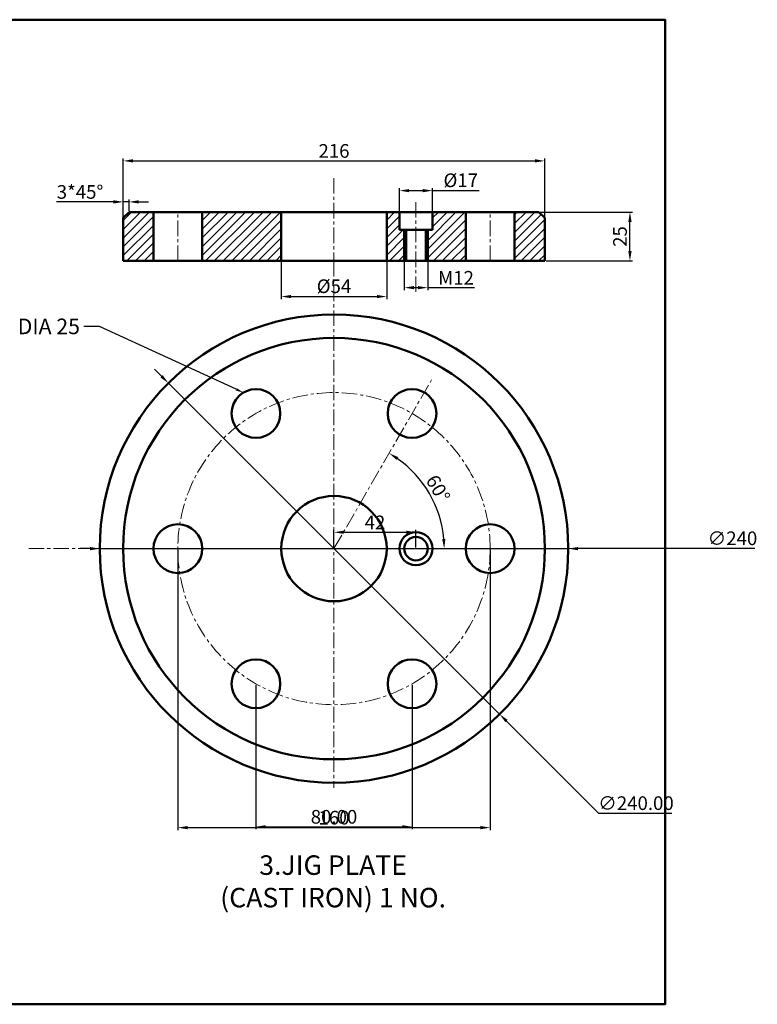
# Model space of a CAD drawing. Units: millimetres. Extents: x 51 to 972, y -225 to 280.
# Tile 3 of 3: x 594 to 972, y -225 to 280. Entities that reach past the tile are written whole.
import ezdxf
from ezdxf import colors
from ezdxf.entities.mleader import LeaderData, LeaderLine
from ezdxf.math import Vec2, Vec3

# ---------------------------------------------------------------- set-up
doc = ezdxf.new("R2010")
doc.units = ezdxf.units.MM
doc.header["$LTSCALE"] = 0.5
doc.linetypes.add('CENTER', pattern=[50.8, 31.75, -6.35, 6.35, -6.35])
for name, color, linetype, lineweight in [('M-CNTR', 1, 'CENTER', 18), ('M-DIMS', 2, 'Continuous', 25), ('M-HATC', 8, 'Continuous', 18), ('M-OUTL', 7, 'Continuous', 50), ('M-TEXT', 7, 'Continuous', 25), ('M-TTLB', 7, 'Continuous', 50)]:
    doc.layers.add(name, color=color, linetype=linetype, lineweight=lineweight)
doc.styles.get("Standard").update_dxf_attribs({"font": 'arial.ttf'})
doc.dimstyles.new('ISO-25', dxfattribs={"dimtxt": 7, "dimasz": 5, "dimexe": 1.25, "dimexo": 0.625, "dimtad": 1, "dimtoh": 1, "dimtxsty": 'Standard', "dimcen": 2.5, "dimadec": 0, "dimazin": 0, "dimtfac": 1, "dimtmove": 0, "dimatfit": 3, "dimfxl": 1, "dimarcsym": 0})

# ---------------------------------------------------------------- blocks, each defined once
blk = doc.blocks.new('*D37')
at = {"layer": 'Defpoints', "color": 0, "ltscale": 0.5, "transparency": 16777216}
for p in [(728.45, 156.09), (782.45, 156.09), (782.45, 137.8)]:
    blk.add_point(p, dxfattribs=at)
at = {"layer": 'M-DIMS', "color": 0, "lineweight": -2, "ltscale": 0.5, "transparency": 16777216}
for p, q in [((728.45, 155.46), (728.45, 136.55)), ((782.45, 155.46), (782.45, 136.55)), ((733.45, 137.8), (777.45, 137.8))]:
    blk.add_line(p, q, dxfattribs=at)
at = {"layer": 'M-DIMS', "color": 0, "ltscale": 0.5, "transparency": 16777216}
for points in [[(733.45, 138.64), (733.45, 136.97), (728.45, 137.8)], [(777.45, 138.64), (777.45, 136.97), (782.45, 137.8)]]:
    blk.add_solid(points, dxfattribs=at)
at = {"layer": 'M-DIMS', "color": 0, "ltscale": 0.5, "transparency": 16777216, "insert": (755.45, 142.2), "char_height": 7, "attachment_point": 5}
blk.add_mtext('%%C54', dxfattribs=at)
blk = doc.blocks.new('*D38')
at = {"layer": 'Defpoints', "color": 0, "ltscale": 0.5, "transparency": 16777216}
for p in [(675.45, 8.59), (835.45, 8.59), (835.45, -134.43)]:
    blk.add_point(p, dxfattribs=at)
at = {"layer": 'M-DIMS', "color": 0, "lineweight": -2, "ltscale": 0.5, "transparency": 16777216}
for p, q in [((675.45, 7.97), (675.45, -135.68)), ((835.45, 7.97), (835.45, -135.68)), ((680.45, -134.43), (830.45, -134.43))]:
    blk.add_line(p, q, dxfattribs=at)
at = {"layer": 'M-DIMS', "color": 0, "ltscale": 0.5, "transparency": 16777216}
for points in [[(680.45, -133.6), (680.45, -135.27), (675.45, -134.43)], [(830.45, -133.6), (830.45, -135.27), (835.45, -134.43)]]:
    blk.add_solid(points, dxfattribs=at)
at = {"layer": 'M-DIMS', "color": 0, "ltscale": 0.5, "transparency": 16777216, "insert": (755.45, -130.23), "char_height": 7, "attachment_point": 5}
blk.add_mtext('160', dxfattribs=at)
blk = doc.blocks.new('*D39')
at = {"layer": 'Defpoints', "color": 0, "ltscale": 0.5, "transparency": 16777216}
for p in [(797.45, 16.98), (755.45, 8.59), (797.45, 8.59)]:
    blk.add_point(p, dxfattribs=at)
at = {"layer": 'M-DIMS', "color": 0, "lineweight": -2, "ltscale": 0.5, "transparency": 16777216}
for p, q in [((755.45, 9.22), (755.45, 18.23)), ((760.45, 16.98), (792.45, 16.98)), ((797.45, 9.22), (797.45, 18.23))]:
    blk.add_line(p, q, dxfattribs=at)
at = {"layer": 'M-DIMS', "color": 0, "ltscale": 0.5, "transparency": 16777216}
for points in [[(760.45, 17.81), (760.45, 16.14), (755.45, 16.98)], [(792.45, 17.81), (792.45, 16.14), (797.45, 16.98)]]:
    blk.add_solid(points, dxfattribs=at)
at = {"layer": 'M-DIMS', "color": 0, "ltscale": 0.5, "transparency": 16777216, "insert": (776.45, 21.12), "char_height": 7, "attachment_point": 5}
blk.add_mtext('42', dxfattribs=at)
blk = doc.blocks.new('*D40')
at = {"layer": 'Defpoints', "color": 0, "ltscale": 0.5, "transparency": 16777216}
for p in [(805.93, 96.03), (808.52, 27.91), (599.02, 8.59), (755.45, 8.59), (887.08, 8.59)]:
    blk.add_point(p, dxfattribs=at)
at = {"layer": 'M-DIMS', "color": 0, "lineweight": -2, "ltscale": 0.5, "transparency": 16777216}
blk.add_arc((755.45, 8.59), 56.47, 5.0746, 54.9254, dxfattribs=at)
at = {"layer": 'M-DIMS', "color": 0, "ltscale": 0.5, "transparency": 16777216}
for points in [[(787.45, 54.11), (788.35, 55.51), (783.69, 57.5)], [(812.53, 13.62), (810.87, 13.55), (811.92, 8.59)]]:
    blk.add_solid(points, dxfattribs=at)
at = {"layer": 'M-DIMS', "color": 0, "ltscale": 0.5, "transparency": 16777216, "insert": (807.99, 38.93), "char_height": 7, "attachment_point": 5, "rotation": 300}
blk.add_mtext('60°', dxfattribs=at)
blk = doc.blocks.new('*D41')
at = {"layer": 'Defpoints', "color": 0, "ltscale": 0.5, "transparency": 16777216}
for p in [(863.45, 207.35), (647.45, 167.09), (863.45, 167.09)]:
    blk.add_point(p, dxfattribs=at)
at = {"layer": 'M-DIMS', "color": 0, "lineweight": -2, "ltscale": 0.5, "transparency": 16777216}
for p, q in [((647.45, 167.71), (647.45, 208.6)), ((652.45, 207.35), (858.45, 207.35)), ((863.45, 167.71), (863.45, 208.6))]:
    blk.add_line(p, q, dxfattribs=at)
at = {"layer": 'M-DIMS', "color": 0, "ltscale": 0.5, "transparency": 16777216}
for points in [[(652.45, 208.19), (652.45, 206.52), (647.45, 207.35)], [(858.45, 208.19), (858.45, 206.52), (863.45, 207.35)]]:
    blk.add_solid(points, dxfattribs=at)
at = {"layer": 'M-DIMS', "color": 0, "ltscale": 0.5, "transparency": 16777216, "insert": (755.45, 211.55), "char_height": 7, "attachment_point": 5}
blk.add_mtext('216', dxfattribs=at)
blk = doc.blocks.new('*D42')
at = {"layer": 'Defpoints', "color": 0, "ltscale": 0.5, "transparency": 16777216}
for p in [(791.45, 156.09), (803.45, 156.09), (803.45, 142.37)]:
    blk.add_point(p, dxfattribs=at)
at = {"layer": 'M-DIMS', "color": 0, "lineweight": -2, "ltscale": 0.5, "transparency": 16777216}
for p, q in [((791.45, 155.46), (791.45, 141.12)), ((803.45, 155.46), (803.45, 141.12)), ((796.45, 142.37), (798.45, 142.37)), ((803.45, 142.37), (827.48, 142.37))]:
    blk.add_line(p, q, dxfattribs=at)
at = {"layer": 'M-DIMS', "color": 0, "ltscale": 0.5, "transparency": 16777216}
for points in [[(796.45, 143.21), (796.45, 141.54), (791.45, 142.37)], [(798.45, 143.21), (798.45, 141.54), (803.45, 142.37)]]:
    blk.add_solid(points, dxfattribs=at)
at = {"layer": 'M-DIMS', "color": 0, "ltscale": 0.5, "transparency": 16777216, "insert": (817.97, 146.51), "char_height": 7, "attachment_point": 5}
blk.add_mtext('M12', dxfattribs=at)
blk = doc.blocks.new('*D43')
at = {"layer": 'Defpoints', "color": 0, "ltscale": 0.5, "transparency": 16777216}
for p in [(805.95, 192.1), (788.95, 181.09), (805.95, 181.09)]:
    blk.add_point(p, dxfattribs=at)
at = {"layer": 'M-DIMS', "color": 0, "lineweight": -2, "ltscale": 0.5, "transparency": 16777216}
for p, q in [((788.95, 181.71), (788.95, 193.35)), ((793.95, 192.1), (800.95, 192.1)), ((805.95, 181.71), (805.95, 193.35)), ((805.95, 192.1), (829.84, 192.1))]:
    blk.add_line(p, q, dxfattribs=at)
at = {"layer": 'M-DIMS', "color": 0, "ltscale": 0.5, "transparency": 16777216}
for points in [[(793.95, 192.93), (793.95, 191.27), (788.95, 192.1)], [(800.95, 192.93), (800.95, 191.27), (805.95, 192.1)]]:
    blk.add_solid(points, dxfattribs=at)
at = {"layer": 'M-DIMS', "color": 0, "ltscale": 0.5, "transparency": 16777216, "insert": (820.4, 196.49), "char_height": 7, "attachment_point": 5}
blk.add_mtext('%%C17', dxfattribs=at)
blk = doc.blocks.new('*D44')
at = {"layer": 'Defpoints', "color": 0, "ltscale": 0.5, "transparency": 16777216}
for p in [(647.45, 186.33), (647.45, 178.09), (650.45, 181.09)]:
    blk.add_point(p, dxfattribs=at)
at = {"layer": 'M-DIMS', "color": 0, "lineweight": -2, "ltscale": 0.5, "transparency": 16777216}
for p, q in [((647.45, 178.71), (647.45, 187.58)), ((650.45, 181.71), (650.45, 187.58)), ((642.45, 186.33), (613.23, 186.33)), ((650.45, 186.33), (647.45, 186.33)), ((655.45, 186.33), (660.45, 186.33))]:
    blk.add_line(p, q, dxfattribs=at)
at = {"layer": 'M-DIMS', "color": 0, "ltscale": 0.5, "transparency": 16777216}
for points in [[(642.45, 187.17), (642.45, 185.5), (647.45, 186.33)], [(655.45, 187.17), (655.45, 185.5), (650.45, 186.33)]]:
    blk.add_solid(points, dxfattribs=at)
at = {"layer": 'M-DIMS', "color": 0, "ltscale": 0.5, "transparency": 16777216, "insert": (625.34, 190.53), "char_height": 7, "attachment_point": 5}
blk.add_mtext('3*45%%D', dxfattribs=at)
blk = doc.blocks.new('*D45')
at = {"layer": 'Defpoints', "color": 0, "ltscale": 0.5, "transparency": 16777216}
for p in [(860.45, 181.09), (907.08, 181.09), (863.45, 156.09)]:
    blk.add_point(p, dxfattribs=at)
at = {"layer": 'M-DIMS', "color": 0, "lineweight": -2, "ltscale": 0.5, "transparency": 16777216}
for p, q in [((861.08, 181.09), (908.33, 181.09)), ((907.08, 161.09), (907.08, 176.09)), ((864.08, 156.09), (908.33, 156.09))]:
    blk.add_line(p, q, dxfattribs=at)
at = {"layer": 'M-DIMS', "color": 0, "ltscale": 0.5, "transparency": 16777216}
for points in [[(906.25, 176.09), (907.92, 176.09), (907.08, 181.09)], [(906.25, 161.09), (907.92, 161.09), (907.08, 156.09)]]:
    blk.add_solid(points, dxfattribs=at)
at = {"layer": 'M-DIMS', "color": 0, "ltscale": 0.5, "transparency": 16777216, "insert": (902.89, 168.59), "char_height": 7, "attachment_point": 5, "rotation": 90}
blk.add_mtext('25', dxfattribs=at)
blk = doc.blocks.new('*D47')
at = {"layer": 'Defpoints', "color": 0, "ltscale": 0.5, "transparency": 16777216}
for p in [(635.45, 8.59), (875.45, 8.59)]:
    blk.add_point(p, dxfattribs=at)
at = {"layer": 'M-DIMS', "color": 0, "lineweight": -2, "ltscale": 0.5, "transparency": 16777216}
for p, q in [((630.45, 8.59), (625.45, 8.59)), ((635.45, 8.59), (875.45, 8.59)), ((947.45, 8.59), (880.45, 8.59)), ((971.13, 8.59), (947.45, 8.59))]:
    blk.add_line(p, q, dxfattribs=at)
at = {"layer": 'M-DIMS', "color": 0, "ltscale": 0.5, "transparency": 16777216}
for points in [[(630.45, 9.42), (630.45, 7.76), (635.45, 8.59)], [(880.45, 9.42), (880.45, 7.76), (875.45, 8.59)]]:
    blk.add_solid(points, dxfattribs=at)
at = {"layer": 'M-DIMS', "color": 0, "ltscale": 0.5, "transparency": 16777216, "insert": (959.6, 12.99), "char_height": 7, "attachment_point": 5}
blk.add_mtext('∅240', dxfattribs=at)
blk = doc.blocks.new('*D59')
at = {"layer": 'Defpoints', "color": 0, "ltscale": 0.5, "transparency": 16777216}
for p in [(715.45, -60.69), (795.45, -60.69), (795.45, -133.98)]:
    blk.add_point(p, dxfattribs=at)
at = {"layer": 'M-DIMS', "color": 0, "lineweight": -2, "ltscale": 0.5, "transparency": 16777216}
for p, q in [((715.45, -61.32), (715.45, -135.23)), ((795.45, -61.32), (795.45, -135.23)), ((720.45, -133.98), (790.45, -133.98))]:
    blk.add_line(p, q, dxfattribs=at)
at = {"layer": 'M-DIMS', "color": 0, "ltscale": 0.5, "transparency": 16777216}
for points in [[(720.45, -133.15), (720.45, -134.81), (715.45, -133.98)], [(790.45, -133.15), (790.45, -134.81), (795.45, -133.98)]]:
    blk.add_solid(points, dxfattribs=at)
at = {"layer": 'M-DIMS', "color": 0, "ltscale": 0.5, "transparency": 16777216, "insert": (755.45, -129.78), "char_height": 7, "attachment_point": 5}
blk.add_mtext('80.00', dxfattribs=at)
blk = doc.blocks.new('*D60')
at = {"layer": 'Defpoints', "color": 0, "ltscale": 0.5, "transparency": 16777216}
for p in [(670.6, 93.45), (840.3, -76.26)]:
    blk.add_point(p, dxfattribs=at)
at = {"layer": 'M-DIMS', "color": 0, "lineweight": -2, "ltscale": 0.5, "transparency": 16777216}
for p, q in [((667.06, 96.98), (663.53, 100.52)), ((670.6, 93.45), (840.3, -76.26)), ((891.21, -127.17), (843.84, -79.8)), ((928.49, -127.17), (891.21, -127.17))]:
    blk.add_line(p, q, dxfattribs=at)
at = {"layer": 'M-DIMS', "color": 0, "ltscale": 0.5, "transparency": 16777216}
for points in [[(667.65, 97.57), (666.47, 96.39), (670.6, 93.45)], [(844.43, -79.21), (843.25, -80.39), (840.3, -76.26)]]:
    blk.add_solid(points, dxfattribs=at)
at = {"layer": 'M-DIMS', "color": 0, "ltscale": 0.5, "transparency": 16777216, "insert": (910.16, -122.78), "char_height": 7, "attachment_point": 5}
blk.add_mtext('∅240.00', dxfattribs=at)

msp = doc.modelspace()

# ---------------------------------------------------------------- hatches: boundary and pattern name
at = {"layer": 'M-HATC', "ltscale": 0.5}
h = msp.add_hatch(dxfattribs=at)
h.set_pattern_fill('ANSI31', color=256)
h.set_pattern_definition([(45, (-59.137, 1e-14), (-2.245064, 2.245064), [])])
h.paths.add_polyline_path([(662.9509, 181.0873), (650.4509, 181.0873), (647.4509, 178.0873), (647.4509, 156.0873), (662.9509, 156.0873)])
h.paths.add_polyline_path([(687.9509, 181.0873), (687.9509, 156.0873), (728.4509, 156.0873), (728.4509, 181.0873)])
h.paths.add_polyline_path([(791.4509, 172.0873), (788.9509, 172.0873), (788.9509, 181.0873), (782.4509, 181.0873), (782.4509, 156.0873), (791.4509, 156.0873)])
h.paths.add_polyline_path([(803.4509, 156.0873), (805.9509, 156.0873), (822.9509, 156.0873), (822.9509, 181.0873), (805.9509, 181.0873), (805.9509, 172.0873), (803.4509, 172.0873)])
h.paths.add_polyline_path([(847.9509, 156.0873), (863.4509, 156.0873), (863.4509, 178.0873), (860.4509, 181.0873), (847.9509, 181.0873)])

# ---------------------------------------------------------------- linework, layer by layer
at = {"layer": 'M-CNTR', "ltscale": 0.5}
for p, q in [((797.4509, 186.2449), (797.4509, 138.622)), ((675.4509, 156.0873), (675.4509, 181.0873)), ((835.4509, 156.0873), (835.4509, 181.0873)), ((755.4509, 8.5913), (805.931, 96.0254)), ((599.0192, 8.5913), (887.0846, 8.5913))]:
    msp.add_line(p, q, dxfattribs=at)
msp.add_lwpolyline([(755.4509, 198.525), (755.4509, 156.0873), (755.4509, -113.9816)], dxfattribs=at)
msp.add_circle((755.4509, 8.5913), 80, dxfattribs=at)
at = {"layer": 'M-OUTL', "ltscale": 0.5}
for p, q in [((650.4509, 181.0873), (647.4509, 178.0873)), ((647.4509, 156.0873), (647.4509, 178.0873)), ((650.4509, 181.0873), (860.4509, 181.0873)), ((662.9509, 156.0873), (662.9509, 181.0873)), ((687.9509, 156.0873), (687.9509, 181.0873)), ((728.4509, 156.0873), (728.4509, 181.0873)), ((755.4509, 181.0873), (845.4509, 181.0873)), ((755.4509, 181.0873), (835.4509, 181.0873)), ((782.4509, 156.0873), (782.4509, 181.0873)), ((788.9509, 181.0873), (788.9509, 172.0873)), ((805.9509, 181.0873), (805.9509, 172.0873)), ((822.9509, 156.0873), (822.9509, 181.0873)), ((847.9509, 156.0873), (847.9509, 181.0873)), ((860.4509, 181.0873), (863.4509, 178.0873)), ((863.4509, 178.0873), (863.4509, 156.0873)), ((788.9509, 172.0873), (805.9509, 172.0873)), ((791.4509, 172.0873), (791.4509, 156.0873)), ((792.4509, 172.0873), (792.4509, 156.0873)), ((802.4509, 172.0873), (802.4509, 156.0873)), ((803.4509, 172.0873), (803.4509, 156.0873)), ((863.4509, 156.0873), (647.4509, 156.0873)), ((788.9509, 156.0873), (805.9509, 156.0873))]:
    msp.add_line(p, q, dxfattribs=at)
for centre, radius in [((755.4509, 8.5913), 120), ((755.4509, 8.5913), 108), ((715.4509, 77.8734), 12.5), ((795.4509, 77.8734), 12.5), ((755.4509, 8.5913), 27), ((675.4509, 8.5913), 12.5), ((835.4509, 8.5913), 12.5), ((797.4509, 8.5913), 8.5), ((797.4509, 8.5913), 6), ((715.4509, -60.6907), 12.5), ((795.4509, -60.6907), 12.5)]:
    msp.add_circle(centre, radius, dxfattribs=at)
at = {"layer": 'M-TTLB', "ltscale": 0.5}
msp.add_lwpolyline([(50.8898, 279.7282), (925.0778, 279.7282), (925.0778, -224.9845), (50.8898, -224.9845)], close=True, dxfattribs=at)

# ---------------------------------------------------------------- texts
at = {"layer": 'M-TEXT', "insert": (659.2905, -148.6313), "char_height": 10, "attachment_point": 1}
msp.add_mtext_dynamic_manual_height_columns('\\pxqc;3.JIG PLATE \\P(CAST IRON) 1 NO. ', width=191.418549, gutter_width=12.5, heights=[0], dxfattribs=at)

# ---------------------------------------------------------------- dimensions: what is measured, and where the dimension line sits
at = {"layer": 'M-DIMS', "ltscale": 0.5}
for base, p1, p2, override, picture, middle in [((863.4509, 207.3532), (647.4509, 167.0873), (863.4509, 167.0873), {"dimclrd": 0, "dimclre": 0, "dimclrt": 0}, '*D41', (755.4509, 211.5522)), ((797.4509, 16.9783), (755.4509, 8.5913), (797.4509, 8.5913), {"dimclrd": 0, "dimclre": 0, "dimclrt": 0}, '*D39', (776.4509, 21.1176)), ((835.4509, -134.4329), (675.4509, 8.5913), (835.4509, 8.5913), {"dimclrd": 0, "dimclre": 0, "dimclrt": 0}, '*D38', (755.4509, -130.2339)), ((795.4509, -133.9816), (715.4509, -60.6907), (795.4509, -60.6907), {"dimdec": 2, "dimlfac": 1, "dimrnd": 0, "dimzin": 0, "dimdsep": 46, "dimlunit": 2}, '*D59', (755.4509, -129.7826))]:
    dim = msp.add_linear_dim(base=base, p1=p1, p2=p2, dimstyle='ISO-25', override=override, dxfattribs=at)
    dim.commit()
    dim.dimension.update_dxf_attribs({"geometry": picture, "text_midpoint": middle})
for base, p1, p2, text, picture, middle in [((805.9509, 192.0986), (788.9509, 181.0873), (805.9509, 181.0873), '%%C<>', '*D43', (820.3976, 196.4933)), ((647.4509, 186.3323), (650.4509, 181.0873), (647.4509, 178.0873), '<>*45%%D', '*D44', (625.3399, 190.5336)), ((782.4509, 137.8041), (728.4509, 156.0873), (782.4509, 156.0873), '%%C<>', '*D37', (755.4509, 142.1989))]:
    dim = msp.add_linear_dim(base=base, p1=p1, p2=p2, text=text, dimstyle='ISO-25', override={"dimclrd": 0, "dimclre": 0, "dimclrt": 0}, dxfattribs=at)
    dim.commit()
    dim.dimension.update_dxf_attribs({"geometry": picture, "text_midpoint": middle})
dim = msp.add_linear_dim(base=(907.0846, 181.0873), p1=(863.4509, 156.0873), p2=(860.4509, 181.0873), angle=90, dimstyle='ISO-25', override={"dimdec": 0, "dimlfac": 1, "dimrnd": 0, "dimzin": 0, "dimdsep": 46, "dimlunit": 2}, dxfattribs=at)
dim.commit()
dim.dimension.update_dxf_attribs({"geometry": '*D45', "text_midpoint": (902.8856, 168.5873)})
dim = msp.add_linear_dim(base=(803.4509, 142.372), p1=(791.4509, 156.0873), p2=(803.4509, 156.0873), text='M<>', dimstyle='ISO-25', override={"dimclrd": 0, "dimclre": 0, "dimclrt": 0}, dxfattribs=at)
dim.commit()
dim.dimension.update_dxf_attribs({"geometry": '*D42', "text_midpoint": (817.9668, 142.372), "dimtype": 160})
dim = msp.add_angular_dim_2l(base=(808.5172, 27.9059), line1=((599.0192, 8.5913), (887.0846, 8.5913)), line2=((755.4509, 8.5913), (805.931, 96.0254)), dimstyle='ISO-25', override={"dimclrd": 0, "dimclre": 0, "dimclrt": 0}, dxfattribs=at)
dim.commit()
dim.dimension.update_dxf_attribs({"geometry": '*D40', "text_midpoint": (807.9935, 38.9268)})
for p1, p2, override, picture, middle in [((670.5993, 93.4453), (840.3026, -76.2626), {"dimdec": 2, "dimlfac": 1, "dimrnd": 0, "dimzin": 0, "dimdsep": 46, "dimlunit": 2}, '*D60', (910.1647, -127.175)), ((635.4509, 8.5916), (875.4509, 8.591), {"dimdec": 0, "dimlfac": 1, "dimrnd": 0, "dimzin": 0, "dimdsep": 46, "dimlunit": 2}, '*D47', (947.4509, 8.5908))]:
    dim = msp.add_diameter_dim_2p(p1=p1, p2=p2, dimstyle='ISO-25', override=override, dxfattribs=at)
    dim.commit()
    dim.dimension.update_dxf_attribs({"geometry": picture, "text_midpoint": middle, "dimtype": 163})

# ---------------------------------------------------------------- leaders
ml = msp.add_multileader_mtext('Standard', dxfattribs=at)
ml.set_content('6 HOLES DIA 25', color=256)
ml.set_leader_properties()
ml.build(insert=Vec2(0, 0))
ctx = ml.context
ctx.base_point, ctx.char_height, ctx.plane_origin = Vec3(539.6854, 122.4495), 8, Vec3(709.0048, 88.583)
ctx.text_align_type = 2
notes = []
notes.append((ctx, [(0, (1, 1, 0), (635.298, 122.4495), (-1, 0), 8, [(0, [(709.0048, 88.583)], 0, [])])]))
ctx.mtext.insert, ctx.mtext.alignment, ctx.mtext.flow_direction = Vec3(625.298, 126.5177), 3, 5
for ctx, leaders in notes:
    for number, flags, end, landing, length, lines in leaders:
        leader = LeaderData()
        leader.index, (leader.has_last_leader_line, leader.has_dogleg_vector, leader.attachment_direction) = number, flags
        leader.last_leader_point, leader.dogleg_vector, leader.dogleg_length = Vec3(end), Vec3(landing), length
        for number, points, colour, breaks in lines:
            line = LeaderLine()
            line.index, line.vertices, line.color, line.breaks = number, Vec3.list(points), colors.encode_raw_color(colour), breaks
            leader.lines.append(line)
        ctx.leaders.append(leader)

doc.saveas('drawing.dxf')
